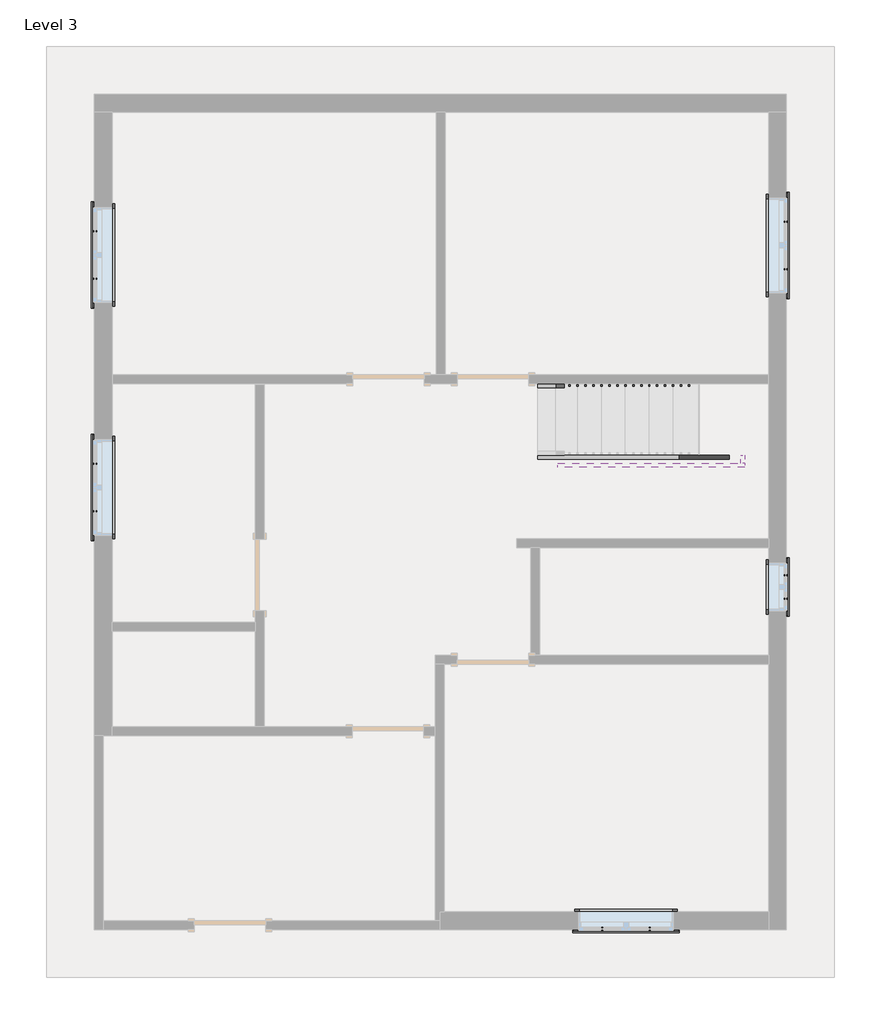
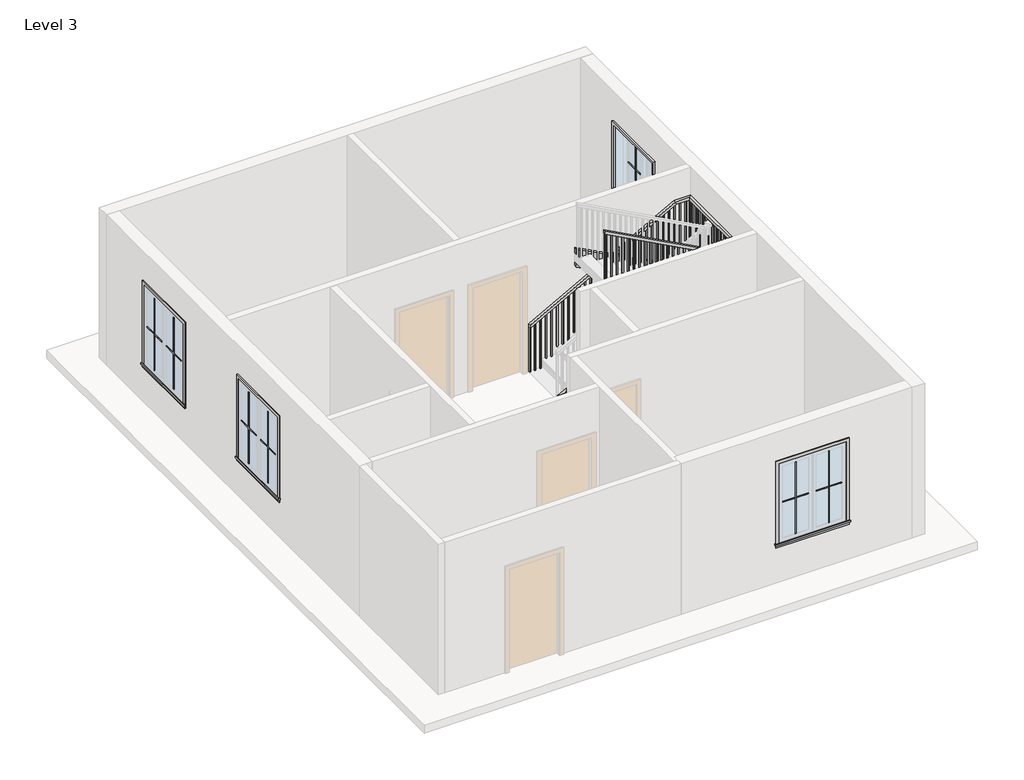
# One storey, part 2 of 2: 20 proxies, 3 members, 1 railing.
"""IFC4 building model written with IfcOpenShell, lengths in millimetres."""

from ifc_helpers import new_model, si_unit, frame, origin, place, context, project, spatial, polyline, outline, extrude, faceted_brep, transform, mapped, element, save
from components import muntin_pattern_2x2_muntin_pattern_2x2_6dad3731, muntin_pattern_2x2_muntin_pattern_2x2_a30a3345, muntin_pattern_2x2_muntin_pattern_2x2_53152e2c, muntin_pattern_2x2_muntin_pattern_2x2_e8f3e573, trim_window_exterior_flat_with_sill_92b9b949, trim_window_exterior_flat_with_sill_a665a915, trim_window_interior_flat_picture_frame_3bb882cf, trim_window_interior_flat_picture_frame_d485c387

model = new_model("IFC4")

# Units and contexts
model_context = context("Model", 3, world=origin())
ifc_project = project(units=[si_unit("LENGTHUNIT", "METRE", prefix="MILLI")], contexts=[model_context])

# Site, building, storey
site = spatial("IfcSite", under=ifc_project)
building = spatial("IfcBuilding", under=site)
storey = spatial("IfcBuildingStorey", under=building, Name="Level 3", Elevation=6096.0)

# Proxies
placement = place(None, origin())
muntin_pattern_2x2_muntin_pattern_2x2_shape = muntin_pattern_2x2_muntin_pattern_2x2_6dad3731(model_context)
element("IfcBuildingElementProxy", 1, Name="Muntin Pattern_2x2 : Muntin Pattern_2x2", ObjectType="Muntin Pattern_2x2 : Muntin Pattern_2x2", at=placement, inside=storey, context=model_context, shape_type="MappedRepresentation", body=[
    mapped(muntin_pattern_2x2_muntin_pattern_2x2_shape, transform((10003.63125, 2232.025, 7080.25), x_axis=(-1.0, 0.0, 0.0), y_axis=(0.0, -1.0, 0.0), z_axis=(0.0, 0.0, 1.0))),
])
element("IfcBuildingElementProxy", 2, Name="Muntin Pattern_2x2 : Muntin Pattern_2x2", ObjectType="Muntin Pattern_2x2 : Muntin Pattern_2x2", at=placement, inside=storey, context=model_context, shape_type="MappedRepresentation", body=[
    mapped(muntin_pattern_2x2_muntin_pattern_2x2_shape, transform((2917.825, 7567.6125, 7080.25), x_axis=(0.0, 1.0, 0.0), y_axis=(-1.0, 0.0, 0.0), z_axis=(0.0, 0.0, 1.0))),
])
element("IfcBuildingElementProxy", 3, Name="Muntin Pattern_2x2 : Muntin Pattern_2x2", ObjectType="Muntin Pattern_2x2 : Muntin Pattern_2x2", at=placement, inside=storey, context=model_context, shape_type="MappedRepresentation", body=[
    mapped(muntin_pattern_2x2_muntin_pattern_2x2_shape, transform((2917.825, 10536.2375, 7080.25), x_axis=(0.0, 1.0, 0.0), y_axis=(-1.0, 0.0, 0.0), z_axis=(0.0, 0.0, 1.0))),
])
element("IfcBuildingElementProxy", 4, Name="Muntin Pattern_2x2 : Muntin Pattern_2x2", ObjectType="Muntin Pattern_2x2 : Muntin Pattern_2x2", at=placement, inside=storey, context=model_context, shape_type="MappedRepresentation", body=[
    mapped(muntin_pattern_2x2_muntin_pattern_2x2_shape, transform((11737.975, 11264.9, 7080.25), x_axis=(0.0, -1.0, 0.0), y_axis=(1.0, 0.0, 0.0), z_axis=(0.0, 0.0, 1.0))),
])
muntin_pattern_2x2_muntin_pattern_2x2_2_shape = muntin_pattern_2x2_muntin_pattern_2x2_a30a3345(model_context)
element("IfcBuildingElementProxy", 5, Name="Muntin Pattern_2x2 : Muntin Pattern_2x2", ObjectType="Muntin Pattern_2x2 : Muntin Pattern_2x2", at=placement, inside=storey, context=model_context, shape_type="MappedRepresentation", body=[
    mapped(muntin_pattern_2x2_muntin_pattern_2x2_2_shape, transform((9397.20625, 2232.025, 7080.25), x_axis=(1.0, 0.0, 0.0), y_axis=(0.0, 1.0, 0.0), z_axis=(0.0, 0.0, 1.0))),
])
element("IfcBuildingElementProxy", 6, Name="Muntin Pattern_2x2 : Muntin Pattern_2x2", ObjectType="Muntin Pattern_2x2 : Muntin Pattern_2x2", at=placement, inside=storey, context=model_context, shape_type="MappedRepresentation", body=[
    mapped(muntin_pattern_2x2_muntin_pattern_2x2_2_shape, transform((2917.825, 8174.0375, 7080.25), x_axis=(0.0, -1.0, 0.0), y_axis=(1.0, 0.0, 0.0), z_axis=(0.0, 0.0, 1.0))),
])
element("IfcBuildingElementProxy", 7, Name="Muntin Pattern_2x2 : Muntin Pattern_2x2", ObjectType="Muntin Pattern_2x2 : Muntin Pattern_2x2", at=placement, inside=storey, context=model_context, shape_type="MappedRepresentation", body=[
    mapped(muntin_pattern_2x2_muntin_pattern_2x2_2_shape, transform((2917.825, 11142.6625, 7080.25), x_axis=(0.0, -1.0, 0.0), y_axis=(1.0, 0.0, 0.0), z_axis=(0.0, 0.0, 1.0))),
])
element("IfcBuildingElementProxy", 8, Name="Muntin Pattern_2x2 : Muntin Pattern_2x2", ObjectType="Muntin Pattern_2x2 : Muntin Pattern_2x2", at=placement, inside=storey, context=model_context, shape_type="MappedRepresentation", body=[
    mapped(muntin_pattern_2x2_muntin_pattern_2x2_2_shape, transform((11737.975, 10658.475, 7080.25), x_axis=(0.0, 1.0, 0.0), y_axis=(-1.0, 0.0, 0.0), z_axis=(0.0, 0.0, 1.0))),
])
muntin_pattern_2x2_muntin_pattern_2x2_3_shape = muntin_pattern_2x2_muntin_pattern_2x2_53152e2c(model_context)
element("IfcBuildingElementProxy", 9, Name="Muntin Pattern_2x2 : Muntin Pattern_2x2", ObjectType="Muntin Pattern_2x2 : Muntin Pattern_2x2", at=placement, inside=storey, context=model_context, shape_type="MappedRepresentation", body=[
    mapped(muntin_pattern_2x2_muntin_pattern_2x2_3_shape, transform((11737.975, 6748.4625, 7080.25), x_axis=(0.0, -1.0, 0.0), y_axis=(1.0, 0.0, 0.0), z_axis=(0.0, 0.0, 1.0))),
])
muntin_pattern_2x2_muntin_pattern_2x2_4_shape = muntin_pattern_2x2_muntin_pattern_2x2_e8f3e573(model_context)
element("IfcBuildingElementProxy", 10, Name="Muntin Pattern_2x2 : Muntin Pattern_2x2", ObjectType="Muntin Pattern_2x2 : Muntin Pattern_2x2", at=placement, inside=storey, context=model_context, shape_type="MappedRepresentation", body=[
    mapped(muntin_pattern_2x2_muntin_pattern_2x2_4_shape, transform((11737.975, 6446.8375, 7080.25), x_axis=(0.0, 1.0, 0.0), y_axis=(-1.0, 0.0, 0.0), z_axis=(0.0, 0.0, 1.0))),
])
trim_window_exterior_flat_with_sill_shape = trim_window_exterior_flat_with_sill_92b9b949(model_context)
element("IfcBuildingElementProxy", 11, Name="Trim-Window-Exterior-Flat : with Sill", ObjectType="Trim-Window-Exterior-Flat : with Sill", at=placement, inside=storey, context=model_context, shape_type="MappedRepresentation", body=[
    mapped(trim_window_exterior_flat_with_sill_shape, transform((9700.41875, 2222.5, 8534.4), x_axis=(1.0, 0.0, 0.0), y_axis=(0.0, 0.0, 1.0), z_axis=(0.0, -1.0, 0.0))),
])
element("IfcBuildingElementProxy", 12, Name="Trim-Window-Exterior-Flat : with Sill", ObjectType="Trim-Window-Exterior-Flat : with Sill", at=placement, inside=storey, context=model_context, shape_type="MappedRepresentation", body=[
    mapped(trim_window_exterior_flat_with_sill_shape, transform((2908.3, 7870.825, 8534.4), x_axis=(0.0, -1.0, 0.0), y_axis=(0.0, 0.0, 1.0), z_axis=(-1.0, 0.0, 0.0))),
])
element("IfcBuildingElementProxy", 13, Name="Trim-Window-Exterior-Flat : with Sill", ObjectType="Trim-Window-Exterior-Flat : with Sill", at=placement, inside=storey, context=model_context, shape_type="MappedRepresentation", body=[
    mapped(trim_window_exterior_flat_with_sill_shape, transform((2908.3, 10839.45, 8534.4), x_axis=(0.0, -1.0, 0.0), y_axis=(0.0, 0.0, 1.0), z_axis=(-1.0, 0.0, 0.0))),
])
element("IfcBuildingElementProxy", 14, Name="Trim-Window-Exterior-Flat : with Sill", ObjectType="Trim-Window-Exterior-Flat : with Sill", at=placement, inside=storey, context=model_context, shape_type="MappedRepresentation", body=[
    mapped(trim_window_exterior_flat_with_sill_shape, transform((11747.5, 10961.6875, 8534.4), x_axis=(0.0, 1.0, 0.0), y_axis=(0.0, 0.0, 1.0), z_axis=(1.0, 0.0, 0.0))),
])
trim_window_exterior_flat_with_sill_2_shape = trim_window_exterior_flat_with_sill_a665a915(model_context)
element("IfcBuildingElementProxy", 15, Name="Trim-Window-Exterior-Flat : with Sill", ObjectType="Trim-Window-Exterior-Flat : with Sill", at=placement, inside=storey, context=model_context, shape_type="MappedRepresentation", body=[
    mapped(trim_window_exterior_flat_with_sill_2_shape, transform((11747.5, 6597.65, 7924.8), x_axis=(0.0, 1.0, 0.0), y_axis=(0.0, 0.0, 1.0), z_axis=(1.0, 0.0, 0.0))),
])
trim_window_interior_flat_picture_frame_shape = trim_window_interior_flat_picture_frame_3bb882cf(model_context)
element("IfcBuildingElementProxy", 16, Name="Trim-Window-Interior-Flat : Picture Frame", ObjectType="Trim-Window-Interior-Flat : Picture Frame", at=placement, inside=storey, context=model_context, shape_type="MappedRepresentation", body=[
    mapped(trim_window_interior_flat_picture_frame_shape, transform((9700.41875, 2451.1, 8534.4), x_axis=(-1.0, 0.0, 0.0), y_axis=(0.0, 0.0, 1.0), z_axis=(0.0, 1.0, 0.0))),
])
element("IfcBuildingElementProxy", 17, Name="Trim-Window-Interior-Flat : Picture Frame", ObjectType="Trim-Window-Interior-Flat : Picture Frame", at=placement, inside=storey, context=model_context, shape_type="MappedRepresentation", body=[
    mapped(trim_window_interior_flat_picture_frame_shape, transform((3136.9, 7870.825, 8534.4), x_axis=(0.0, 1.0, 0.0), y_axis=(0.0, 0.0, 1.0), z_axis=(1.0, 0.0, 0.0))),
])
element("IfcBuildingElementProxy", 18, Name="Trim-Window-Interior-Flat : Picture Frame", ObjectType="Trim-Window-Interior-Flat : Picture Frame", at=placement, inside=storey, context=model_context, shape_type="MappedRepresentation", body=[
    mapped(trim_window_interior_flat_picture_frame_shape, transform((3136.9, 10839.45, 8534.4), x_axis=(0.0, 1.0, 0.0), y_axis=(0.0, 0.0, 1.0), z_axis=(1.0, 0.0, 0.0))),
])
element("IfcBuildingElementProxy", 19, Name="Trim-Window-Interior-Flat : Picture Frame", ObjectType="Trim-Window-Interior-Flat : Picture Frame", at=placement, inside=storey, context=model_context, shape_type="MappedRepresentation", body=[
    mapped(trim_window_interior_flat_picture_frame_shape, transform((11518.9, 10961.6875, 8534.4), x_axis=(0.0, -1.0, 0.0), y_axis=(0.0, 0.0, 1.0), z_axis=(-1.0, 0.0, 0.0))),
])
trim_window_interior_flat_picture_frame_2_shape = trim_window_interior_flat_picture_frame_d485c387(model_context)
element("IfcBuildingElementProxy", 20, Name="Trim-Window-Interior-Flat : Picture Frame", ObjectType="Trim-Window-Interior-Flat : Picture Frame", at=placement, inside=storey, context=model_context, shape_type="MappedRepresentation", body=[
    mapped(trim_window_interior_flat_picture_frame_2_shape, transform((11518.9, 6597.65, 7924.8), x_axis=(0.0, -1.0, 0.0), y_axis=(0.0, 0.0, 1.0), z_axis=(-1.0, 0.0, 0.0))),
])

# Members
element("IfcMember", 21, ObjectType="Stringer - 2\" Width", at=placement, inside=storey, context=model_context, shape_type="SweptSolid", body=[
    extrude(outline(polyline([(6340.4581083, 8572.5), (6096.0, 8572.5), (6096.0, 8761.9689927), (7373.1621978, 11163.3), (7718.3905183, 11163.3), (6340.4581083, 8572.5)])), frame((0.0, 8229.6, 0.0), z_axis=(0.0, 1.0, 0.0), x_axis=(0.0, 0.0, 1.0)), (0.0, 0.0, 1.0), 50.8),
])
element("IfcMember", 22, ObjectType="Stringer - 2\" Width", at=placement, inside=storey, context=model_context, shape_type="SweptSolid", body=[
    extrude(outline(polyline([(11163.3, 8280.4), (11214.1, 8280.4), (11214.1, 8178.8), (11163.3, 8178.8), (11163.3, 8280.4)])), frame((0.0, 0.0, 7471.6105263), z_axis=(0.0, 0.0, 1.0), x_axis=(1.0, 0.0, 0.0)), (0.0, 0.0, 1.0), 304.8),
])
element("IfcMember", 23, ObjectType="Stringer - 2\" Width", at=placement, inside=storey, context=model_context, shape_type="SweptSolid", body=[
    extrude(outline(polyline([(7560.9419568, 11214.1), (7905.380564, 11214.1), (9162.012143, 8826.5), (8817.5735358, 8826.5), (7560.9419568, 11214.1)])), frame((0.0, 8128.0, 0.0), z_axis=(0.0, 1.0, 0.0), x_axis=(0.0, 0.0, 1.0)), (0.0, 0.0, 1.0), 50.8),
])

# Railing
element("IfcRailing", 24, ObjectType="Handrail - Rectangular", at=placement, inside=storey, context=model_context, shape_type="SolidModel", body=[
    faceted_brep([(8572.5, 9194.8, 7170.8210526), (8572.5, 9194.8, 7112.9285199), (8572.5, 9144.0, 7112.9285199), (8572.5, 9144.0, 7170.8210526), (11214.1, 9194.8, 8614.6105263), (11227.076708, 9194.8, 8563.8105263), (11227.076708, 9144.0, 8563.8105263), (11214.1, 9144.0, 8614.6105263), (11518.9, 9194.8, 8614.6105263), (11518.9, 9194.8, 8563.8105263), (11468.1, 9144.0, 8563.8105263), (11468.1, 9144.0, 8614.6105263), (11518.9, 7340.6, 8614.6105263), (11518.9, 7289.8, 8563.8105263), (11468.1, 7289.8, 8563.8105263), (11468.1, 7340.6, 8614.6105263), (11518.9, 7340.6, 8679.4615901), (11518.9, 7289.8, 8628.6615901), (11468.1, 7289.8, 8628.6615901), (11468.1, 7340.6, 8679.4615901), (11518.9, 7213.6, 8679.4615901), (11518.9, 7213.6, 8628.6615901), (11468.1, 7264.4, 8628.6615901), (11468.1, 7264.4, 8679.4615901), (11391.9, 7213.6, 8679.4615901), (11379.1122768, 7213.6, 8628.6615901), (11379.1122768, 7264.4, 8628.6615901), (11391.9, 7264.4, 8679.4615901), (8826.5, 7213.6, 10058.4), (8826.5, 7264.4, 10058.4), (8826.5, 7264.4, 10000.7264198), (8826.5, 7213.6, 10000.7264198)], [[[0, 1, 2, 3]], [[1, 0, 4, 5]], [[2, 1, 5, 6]], [[3, 2, 6, 7]], [[0, 3, 7, 4]], [[5, 4, 8, 9]], [[6, 5, 9, 10]], [[7, 6, 10, 11]], [[4, 7, 11, 8]], [[9, 8, 12, 13]], [[10, 9, 13, 14]], [[11, 10, 14, 15]], [[8, 11, 15, 12]], [[13, 12, 16, 17]], [[14, 13, 17, 18]], [[15, 14, 18, 19]], [[12, 15, 19, 16]], [[17, 16, 20, 21]], [[18, 17, 21, 22]], [[19, 18, 22, 23]], [[16, 19, 23, 20]], [[21, 20, 24, 25]], [[22, 21, 25, 26]], [[23, 22, 26, 27]], [[20, 23, 27, 24]], [[28, 29, 30, 31]], [[25, 24, 28, 31]], [[26, 25, 31, 30]], [[27, 26, 30, 29]], [[24, 27, 29, 28]]]),
    extrude(outline(polyline([(9992.193385, 8842.375), (8983.5789474, 8842.375), (8983.5789474, 8861.425), (9981.9537434, 8861.425), (9992.193385, 8842.375)])), frame((0.0, 7229.475, 0.0), z_axis=(0.0, 1.0, 0.0), x_axis=(0.0, 0.0, 1.0)), (0.0, 0.0, 1.0), 19.05),
    extrude(outline(polyline([(9937.5819629, 8943.975), (8983.5789474, 8943.975), (8983.5789474, 8963.025), (9927.3423212, 8963.025), (9937.5819629, 8943.975)])), frame((0.0, 7229.475, 0.0), z_axis=(0.0, 1.0, 0.0), x_axis=(0.0, 0.0, 1.0)), (0.0, 0.0, 1.0), 19.05),
    extrude(outline(polyline([(9882.9705407, 9045.575), (8983.5789474, 9045.575), (8983.5789474, 9064.625), (9872.730899, 9064.625), (9882.9705407, 9045.575)])), frame((0.0, 7229.475, 0.0), z_axis=(0.0, 1.0, 0.0), x_axis=(0.0, 0.0, 1.0)), (0.0, 0.0, 1.0), 19.05),
    extrude(outline(polyline([(9828.3591185, 9147.175), (8823.1578947, 9147.175), (8823.1578947, 9166.225), (9818.1194769, 9166.225), (9828.3591185, 9147.175)])), frame((0.0, 7229.475, 0.0), z_axis=(0.0, 1.0, 0.0), x_axis=(0.0, 0.0, 1.0)), (0.0, 0.0, 1.0), 19.05),
    extrude(outline(polyline([(9773.7476964, 9248.775), (8823.1578947, 9248.775), (8823.1578947, 9267.825), (9763.5080547, 9267.825), (9773.7476964, 9248.775)])), frame((0.0, 7229.475, 0.0), z_axis=(0.0, 1.0, 0.0), x_axis=(0.0, 0.0, 1.0)), (0.0, 0.0, 1.0), 19.05),
    extrude(outline(polyline([(9719.1362742, 9350.375), (8823.1578947, 9350.375), (8823.1578947, 9369.425), (9708.8966325, 9369.425), (9719.1362742, 9350.375)])), frame((0.0, 7229.475, 0.0), z_axis=(0.0, 1.0, 0.0), x_axis=(0.0, 0.0, 1.0)), (0.0, 0.0, 1.0), 19.05),
    extrude(outline(polyline([(9664.524852, 9451.975), (8662.7368421, 9451.975), (8662.7368421, 9471.025), (9654.2852104, 9471.025), (9664.524852, 9451.975)])), frame((0.0, 7229.475, 0.0), z_axis=(0.0, 1.0, 0.0), x_axis=(0.0, 0.0, 1.0)), (0.0, 0.0, 1.0), 19.05),
    extrude(outline(polyline([(9609.9134298, 9553.575), (8662.7368421, 9553.575), (8662.7368421, 9572.625), (9599.6737882, 9572.625), (9609.9134298, 9553.575)])), frame((0.0, 7229.475, 0.0), z_axis=(0.0, 1.0, 0.0), x_axis=(0.0, 0.0, 1.0)), (0.0, 0.0, 1.0), 19.05),
    extrude(outline(polyline([(9555.3004835, 9655.175), (8662.7368421, 9655.175), (8662.7368421, 9674.225), (9544.8885402, 9674.225), (9555.3004835, 9655.175)])), frame((0.0, 7229.475, 0.0), z_axis=(0.0, 1.0, 0.0), x_axis=(0.0, 0.0, 1.0)), (0.0, 0.0, 1.0), 19.05),
    extrude(outline(polyline([(9500.6905855, 9756.775), (8502.3157895, 9756.775), (8502.3157895, 9775.825), (9490.4509438, 9775.825), (9500.6905855, 9756.775)])), frame((0.0, 7229.475, 0.0), z_axis=(0.0, 1.0, 0.0), x_axis=(0.0, 0.0, 1.0)), (0.0, 0.0, 1.0), 19.05),
    extrude(outline(polyline([(9446.0791633, 9858.375), (8502.3157895, 9858.375), (8502.3157895, 9877.425), (9435.8395217, 9877.425), (9446.0791633, 9858.375)])), frame((0.0, 7229.475, 0.0), z_axis=(0.0, 1.0, 0.0), x_axis=(0.0, 0.0, 1.0)), (0.0, 0.0, 1.0), 19.05),
    extrude(outline(polyline([(9391.4677411, 9959.975), (8502.3157895, 9959.975), (8502.3157895, 9979.025), (9381.2280995, 9979.025), (9391.4677411, 9959.975)])), frame((0.0, 7229.475, 0.0), z_axis=(0.0, 1.0, 0.0), x_axis=(0.0, 0.0, 1.0)), (0.0, 0.0, 1.0), 19.05),
    extrude(outline(polyline([(9336.856319, 10061.575), (8341.8947368, 10061.575), (8341.8947368, 10080.625), (9326.6166773, 10080.625), (9336.856319, 10061.575)])), frame((0.0, 7229.475, 0.0), z_axis=(0.0, 1.0, 0.0), x_axis=(0.0, 0.0, 1.0)), (0.0, 0.0, 1.0), 19.05),
    extrude(outline(polyline([(9282.2448968, 10163.175), (8341.8947368, 10163.175), (8341.8947368, 10182.225), (9272.0052551, 10182.225), (9282.2448968, 10163.175)])), frame((0.0, 7229.475, 0.0), z_axis=(0.0, 1.0, 0.0), x_axis=(0.0, 0.0, 1.0)), (0.0, 0.0, 1.0), 19.05),
    extrude(outline(polyline([(9227.6334746, 10264.775), (8341.8947368, 10264.775), (8341.8947368, 10283.825), (9217.393833, 10283.825), (9227.6334746, 10264.775)])), frame((0.0, 7229.475, 0.0), z_axis=(0.0, 1.0, 0.0), x_axis=(0.0, 0.0, 1.0)), (0.0, 0.0, 1.0), 19.05),
    extrude(outline(polyline([(9173.0220525, 10366.375), (8181.4736842, 10366.375), (8181.4736842, 10385.425), (9162.7824108, 10385.425), (9173.0220525, 10366.375)])), frame((0.0, 7229.475, 0.0), z_axis=(0.0, 1.0, 0.0), x_axis=(0.0, 0.0, 1.0)), (0.0, 0.0, 1.0), 19.05),
    extrude(outline(polyline([(9118.4106303, 10467.975), (8181.4736842, 10467.975), (8181.4736842, 10487.025), (9108.1709886, 10487.025), (9118.4106303, 10467.975)])), frame((0.0, 7229.475, 0.0), z_axis=(0.0, 1.0, 0.0), x_axis=(0.0, 0.0, 1.0)), (0.0, 0.0, 1.0), 19.05),
    extrude(outline(polyline([(9063.7992081, 10569.575), (8181.4736842, 10569.575), (8181.4736842, 10588.625), (9053.5595665, 10588.625), (9063.7992081, 10569.575)])), frame((0.0, 7229.475, 0.0), z_axis=(0.0, 1.0, 0.0), x_axis=(0.0, 0.0, 1.0)), (0.0, 0.0, 1.0), 19.05),
    extrude(outline(polyline([(9009.1877859, 10671.175), (8021.0526316, 10671.175), (8021.0526316, 10690.225), (8998.9481443, 10690.225), (9009.1877859, 10671.175)])), frame((0.0, 7229.475, 0.0), z_axis=(0.0, 1.0, 0.0), x_axis=(0.0, 0.0, 1.0)), (0.0, 0.0, 1.0), 19.05),
    extrude(outline(polyline([(8954.5763638, 10772.775), (8021.0526316, 10772.775), (8021.0526316, 10791.825), (8944.3367221, 10791.825), (8954.5763638, 10772.775)])), frame((0.0, 7229.475, 0.0), z_axis=(0.0, 1.0, 0.0), x_axis=(0.0, 0.0, 1.0)), (0.0, 0.0, 1.0), 19.05),
    extrude(outline(polyline([(8899.9649416, 10874.375), (8021.0526316, 10874.375), (8021.0526316, 10893.425), (8889.7252999, 10893.425), (8899.9649416, 10874.375)])), frame((0.0, 7229.475, 0.0), z_axis=(0.0, 1.0, 0.0), x_axis=(0.0, 0.0, 1.0)), (0.0, 0.0, 1.0), 19.05),
    extrude(outline(polyline([(8845.3535194, 10975.975), (7860.6315789, 10975.975), (7860.6315789, 10995.025), (8835.1138778, 10995.025), (8845.3535194, 10975.975)])), frame((0.0, 7229.475, 0.0), z_axis=(0.0, 1.0, 0.0), x_axis=(0.0, 0.0, 1.0)), (0.0, 0.0, 1.0), 19.05),
    extrude(outline(polyline([(8790.7420972, 11077.575), (7860.6315789, 11077.575), (7860.6315789, 11096.625), (8780.5024556, 11096.625), (8790.7420972, 11077.575)])), frame((0.0, 7229.475, 0.0), z_axis=(0.0, 1.0, 0.0), x_axis=(0.0, 0.0, 1.0)), (0.0, 0.0, 1.0), 19.05),
    extrude(outline(polyline([(8736.1306751, 11179.175), (7860.6315789, 11179.175), (7860.6315789, 11198.225), (8725.8910334, 11198.225), (8736.1306751, 11179.175)])), frame((0.0, 7229.475, 0.0), z_axis=(0.0, 1.0, 0.0), x_axis=(0.0, 0.0, 1.0)), (0.0, 0.0, 1.0), 19.05),
    extrude(outline(polyline([(8681.5192529, 11280.775), (7700.2105263, 11280.775), (7700.2105263, 11299.825), (8671.2796112, 11299.825), (8681.5192529, 11280.775)])), frame((0.0, 7229.475, 0.0), z_axis=(0.0, 1.0, 0.0), x_axis=(0.0, 0.0, 1.0)), (0.0, 0.0, 1.0), 19.05),
    extrude(outline(polyline([(8626.9078307, 11382.375), (7700.2105263, 11382.375), (7700.2105263, 11401.425), (8616.6681891, 11401.425), (8626.9078307, 11382.375)])), frame((0.0, 7229.475, 0.0), z_axis=(0.0, 1.0, 0.0), x_axis=(0.0, 0.0, 1.0)), (0.0, 0.0, 1.0), 19.05),
    extrude(outline(polyline([(11503.025, 7350.125), (11503.025, 7331.075), (11483.975, 7331.075), (11483.975, 7350.125), (11503.025, 7350.125)])), frame((0.0, 0.0, 7700.2105263), z_axis=(0.0, 0.0, 1.0), x_axis=(1.0, 0.0, 0.0)), (0.0, 0.0, 1.0), 863.6),
    extrude(outline(polyline([(11503.025, 7451.725), (11503.025, 7432.675), (11483.975, 7432.675), (11483.975, 7451.725), (11503.025, 7451.725)])), frame((0.0, 0.0, 7700.2105263), z_axis=(0.0, 0.0, 1.0), x_axis=(1.0, 0.0, 0.0)), (0.0, 0.0, 1.0), 863.6),
    extrude(outline(polyline([(11503.025, 7553.325), (11503.025, 7534.275), (11483.975, 7534.275), (11483.975, 7553.325), (11503.025, 7553.325)])), frame((0.0, 0.0, 7700.2105263), z_axis=(0.0, 0.0, 1.0), x_axis=(1.0, 0.0, 0.0)), (0.0, 0.0, 1.0), 863.6),
    extrude(outline(polyline([(11503.025, 7654.925), (11503.025, 7635.875), (11483.975, 7635.875), (11483.975, 7654.925), (11503.025, 7654.925)])), frame((0.0, 0.0, 7700.2105263), z_axis=(0.0, 0.0, 1.0), x_axis=(1.0, 0.0, 0.0)), (0.0, 0.0, 1.0), 863.6),
    extrude(outline(polyline([(11503.025, 7756.525), (11503.025, 7737.475), (11483.975, 7737.475), (11483.975, 7756.525), (11503.025, 7756.525)])), frame((0.0, 0.0, 7700.2105263), z_axis=(0.0, 0.0, 1.0), x_axis=(1.0, 0.0, 0.0)), (0.0, 0.0, 1.0), 863.6),
    extrude(outline(polyline([(11503.025, 7858.125), (11503.025, 7839.075), (11483.975, 7839.075), (11483.975, 7858.125), (11503.025, 7858.125)])), frame((0.0, 0.0, 7700.2105263), z_axis=(0.0, 0.0, 1.0), x_axis=(1.0, 0.0, 0.0)), (0.0, 0.0, 1.0), 863.6),
    extrude(outline(polyline([(11503.025, 7959.725), (11503.025, 7940.675), (11483.975, 7940.675), (11483.975, 7959.725), (11503.025, 7959.725)])), frame((0.0, 0.0, 7700.2105263), z_axis=(0.0, 0.0, 1.0), x_axis=(1.0, 0.0, 0.0)), (0.0, 0.0, 1.0), 863.6),
    extrude(outline(polyline([(11503.025, 8061.325), (11503.025, 8042.275), (11483.975, 8042.275), (11483.975, 8061.325), (11503.025, 8061.325)])), frame((0.0, 0.0, 7700.2105263), z_axis=(0.0, 0.0, 1.0), x_axis=(1.0, 0.0, 0.0)), (0.0, 0.0, 1.0), 863.6),
    extrude(outline(polyline([(11503.025, 8162.925), (11503.025, 8143.875), (11483.975, 8143.875), (11483.975, 8162.925), (11503.025, 8162.925)])), frame((0.0, 0.0, 7700.2105263), z_axis=(0.0, 0.0, 1.0), x_axis=(1.0, 0.0, 0.0)), (0.0, 0.0, 1.0), 863.6),
    extrude(outline(polyline([(11503.025, 8264.525), (11503.025, 8245.475), (11483.975, 8245.475), (11483.975, 8264.525), (11503.025, 8264.525)])), frame((0.0, 0.0, 7700.2105263), z_axis=(0.0, 0.0, 1.0), x_axis=(1.0, 0.0, 0.0)), (0.0, 0.0, 1.0), 863.6),
    extrude(outline(polyline([(11503.025, 8366.125), (11503.025, 8347.075), (11483.975, 8347.075), (11483.975, 8366.125), (11503.025, 8366.125)])), frame((0.0, 0.0, 7700.2105263), z_axis=(0.0, 0.0, 1.0), x_axis=(1.0, 0.0, 0.0)), (0.0, 0.0, 1.0), 863.6),
    extrude(outline(polyline([(11503.025, 8467.725), (11503.025, 8448.675), (11483.975, 8448.675), (11483.975, 8467.725), (11503.025, 8467.725)])), frame((0.0, 0.0, 7700.2105263), z_axis=(0.0, 0.0, 1.0), x_axis=(1.0, 0.0, 0.0)), (0.0, 0.0, 1.0), 863.6),
    extrude(outline(polyline([(11503.025, 8569.325), (11503.025, 8550.275), (11483.975, 8550.275), (11483.975, 8569.325), (11503.025, 8569.325)])), frame((0.0, 0.0, 7700.2105263), z_axis=(0.0, 0.0, 1.0), x_axis=(1.0, 0.0, 0.0)), (0.0, 0.0, 1.0), 863.6),
    extrude(outline(polyline([(11503.025, 8670.925), (11503.025, 8651.875), (11483.975, 8651.875), (11483.975, 8670.925), (11503.025, 8670.925)])), frame((0.0, 0.0, 7700.2105263), z_axis=(0.0, 0.0, 1.0), x_axis=(1.0, 0.0, 0.0)), (0.0, 0.0, 1.0), 863.6),
    extrude(outline(polyline([(11503.025, 8772.525), (11503.025, 8753.475), (11483.975, 8753.475), (11483.975, 8772.525), (11503.025, 8772.525)])), frame((0.0, 0.0, 7700.2105263), z_axis=(0.0, 0.0, 1.0), x_axis=(1.0, 0.0, 0.0)), (0.0, 0.0, 1.0), 863.6),
    extrude(outline(polyline([(11503.025, 8874.125), (11503.025, 8855.075), (11483.975, 8855.075), (11483.975, 8874.125), (11503.025, 8874.125)])), frame((0.0, 0.0, 7700.2105263), z_axis=(0.0, 0.0, 1.0), x_axis=(1.0, 0.0, 0.0)), (0.0, 0.0, 1.0), 863.6),
    extrude(outline(polyline([(11503.025, 8975.725), (11503.025, 8956.675), (11483.975, 8956.675), (11483.975, 8975.725), (11503.025, 8975.725)])), frame((0.0, 0.0, 7700.2105263), z_axis=(0.0, 0.0, 1.0), x_axis=(1.0, 0.0, 0.0)), (0.0, 0.0, 1.0), 863.6),
    extrude(outline(polyline([(11503.025, 9077.325), (11503.025, 9058.275), (11483.975, 9058.275), (11483.975, 9077.325), (11503.025, 9077.325)])), frame((0.0, 0.0, 7700.2105263), z_axis=(0.0, 0.0, 1.0), x_axis=(1.0, 0.0, 0.0)), (0.0, 0.0, 1.0), 863.6),
    extrude(outline(polyline([(11407.775, 9178.925), (11426.825, 9178.925), (11426.825, 9159.875), (11407.775, 9159.875), (11407.775, 9178.925)])), frame((0.0, 0.0, 7700.2105263), z_axis=(0.0, 0.0, 1.0), x_axis=(1.0, 0.0, 0.0)), (0.0, 0.0, 1.0), 863.6),
    extrude(outline(polyline([(11306.175, 9178.925), (11325.225, 9178.925), (11325.225, 9159.875), (11306.175, 9159.875), (11306.175, 9178.925)])), frame((0.0, 0.0, 7700.2105263), z_axis=(0.0, 0.0, 1.0), x_axis=(1.0, 0.0, 0.0)), (0.0, 0.0, 1.0), 863.6),
    extrude(outline(polyline([(8551.512022, 11204.575), (7700.2105263, 11204.575), (7700.2105263, 11223.625), (8561.9239653, 11223.625), (8551.512022, 11204.575)])), frame((0.0, 9159.875, 0.0), z_axis=(0.0, 1.0, 0.0), x_axis=(0.0, 0.0, 1.0)), (0.0, 0.0, 1.0), 19.05),
    extrude(outline(polyline([(8495.9816576, 11102.975), (7539.7894737, 11102.975), (7539.7894737, 11122.025), (8506.3936009, 11122.025), (8495.9816576, 11102.975)])), frame((0.0, 9159.875, 0.0), z_axis=(0.0, 1.0, 0.0), x_axis=(0.0, 0.0, 1.0)), (0.0, 0.0, 1.0), 19.05),
    extrude(outline(polyline([(8440.4512932, 11001.375), (7539.7894737, 11001.375), (7539.7894737, 11020.425), (8450.8632365, 11020.425), (8440.4512932, 11001.375)])), frame((0.0, 9159.875, 0.0), z_axis=(0.0, 1.0, 0.0), x_axis=(0.0, 0.0, 1.0)), (0.0, 0.0, 1.0), 19.05),
    extrude(outline(polyline([(8384.9209288, 10899.775), (7539.7894737, 10899.775), (7539.7894737, 10918.825), (8395.3328722, 10918.825), (8384.9209288, 10899.775)])), frame((0.0, 9159.875, 0.0), z_axis=(0.0, 1.0, 0.0), x_axis=(0.0, 0.0, 1.0)), (0.0, 0.0, 1.0), 19.05),
    extrude(outline(polyline([(8329.3905645, 10798.175), (7379.3684211, 10798.175), (7379.3684211, 10817.225), (8339.8025078, 10817.225), (8329.3905645, 10798.175)])), frame((0.0, 9159.875, 0.0), z_axis=(0.0, 1.0, 0.0), x_axis=(0.0, 0.0, 1.0)), (0.0, 0.0, 1.0), 19.05),
    extrude(outline(polyline([(8273.8602001, 10696.575), (7379.3684211, 10696.575), (7379.3684211, 10715.625), (8284.2721434, 10715.625), (8273.8602001, 10696.575)])), frame((0.0, 9159.875, 0.0), z_axis=(0.0, 1.0, 0.0), x_axis=(0.0, 0.0, 1.0)), (0.0, 0.0, 1.0), 19.05),
    extrude(outline(polyline([(8218.3298357, 10594.975), (7379.3684211, 10594.975), (7379.3684211, 10614.025), (8228.741779, 10614.025), (8218.3298357, 10594.975)])), frame((0.0, 9159.875, 0.0), z_axis=(0.0, 1.0, 0.0), x_axis=(0.0, 0.0, 1.0)), (0.0, 0.0, 1.0), 19.05),
    extrude(outline(polyline([(8162.7994714, 10493.375), (7218.9473684, 10493.375), (7218.9473684, 10512.425), (8173.2114147, 10512.425), (8162.7994714, 10493.375)])), frame((0.0, 9159.875, 0.0), z_axis=(0.0, 1.0, 0.0), x_axis=(0.0, 0.0, 1.0)), (0.0, 0.0, 1.0), 19.05),
    extrude(outline(polyline([(8107.269107, 10391.775), (7218.9473684, 10391.775), (7218.9473684, 10410.825), (8117.6810503, 10410.825), (8107.269107, 10391.775)])), frame((0.0, 9159.875, 0.0), z_axis=(0.0, 1.0, 0.0), x_axis=(0.0, 0.0, 1.0)), (0.0, 0.0, 1.0), 19.05),
    extrude(outline(polyline([(8051.7387426, 10290.175), (7218.9473684, 10290.175), (7218.9473684, 10309.225), (8062.1506859, 10309.225), (8051.7387426, 10290.175)])), frame((0.0, 9159.875, 0.0), z_axis=(0.0, 1.0, 0.0), x_axis=(0.0, 0.0, 1.0)), (0.0, 0.0, 1.0), 19.05),
    extrude(outline(polyline([(7996.2083782, 10188.575), (7058.5263158, 10188.575), (7058.5263158, 10207.625), (8006.6203216, 10207.625), (7996.2083782, 10188.575)])), frame((0.0, 9159.875, 0.0), z_axis=(0.0, 1.0, 0.0), x_axis=(0.0, 0.0, 1.0)), (0.0, 0.0, 1.0), 19.05),
    extrude(outline(polyline([(7940.6780139, 10086.975), (7058.5263158, 10086.975), (7058.5263158, 10106.025), (7951.0899572, 10106.025), (7940.6780139, 10086.975)])), frame((0.0, 9159.875, 0.0), z_axis=(0.0, 1.0, 0.0), x_axis=(0.0, 0.0, 1.0)), (0.0, 0.0, 1.0), 19.05),
    extrude(outline(polyline([(7885.1476495, 9985.375), (7058.5263158, 9985.375), (7058.5263158, 10004.425), (7895.5595928, 10004.425), (7885.1476495, 9985.375)])), frame((0.0, 9159.875, 0.0), z_axis=(0.0, 1.0, 0.0), x_axis=(0.0, 0.0, 1.0)), (0.0, 0.0, 1.0), 19.05),
    extrude(outline(polyline([(7829.6172851, 9883.775), (6898.1052632, 9883.775), (6898.1052632, 9902.825), (7840.0292284, 9902.825), (7829.6172851, 9883.775)])), frame((0.0, 9159.875, 0.0), z_axis=(0.0, 1.0, 0.0), x_axis=(0.0, 0.0, 1.0)), (0.0, 0.0, 1.0), 19.05),
    extrude(outline(polyline([(7774.0869207, 9782.175), (6898.1052632, 9782.175), (6898.1052632, 9801.225), (7784.4988641, 9801.225), (7774.0869207, 9782.175)])), frame((0.0, 9159.875, 0.0), z_axis=(0.0, 1.0, 0.0), x_axis=(0.0, 0.0, 1.0)), (0.0, 0.0, 1.0), 19.05),
    extrude(outline(polyline([(7718.5565564, 9680.575), (6898.1052632, 9680.575), (6898.1052632, 9699.625), (7728.9684997, 9699.625), (7718.5565564, 9680.575)])), frame((0.0, 9159.875, 0.0), z_axis=(0.0, 1.0, 0.0), x_axis=(0.0, 0.0, 1.0)), (0.0, 0.0, 1.0), 19.05),
    extrude(outline(polyline([(7663.026192, 9578.975), (6737.6842105, 9578.975), (6737.6842105, 9598.025), (7673.4381353, 9598.025), (7663.026192, 9578.975)])), frame((0.0, 9159.875, 0.0), z_axis=(0.0, 1.0, 0.0), x_axis=(0.0, 0.0, 1.0)), (0.0, 0.0, 1.0), 19.05),
    extrude(outline(polyline([(7607.4958276, 9477.375), (6737.6842105, 9477.375), (6737.6842105, 9496.425), (7617.9077709, 9496.425), (7607.4958276, 9477.375)])), frame((0.0, 9159.875, 0.0), z_axis=(0.0, 1.0, 0.0), x_axis=(0.0, 0.0, 1.0)), (0.0, 0.0, 1.0), 19.05),
    extrude(outline(polyline([(7551.9654633, 9375.775), (6737.6842105, 9375.775), (6737.6842105, 9394.825), (7562.3774066, 9394.825), (7551.9654633, 9375.775)])), frame((0.0, 9159.875, 0.0), z_axis=(0.0, 1.0, 0.0), x_axis=(0.0, 0.0, 1.0)), (0.0, 0.0, 1.0), 19.05),
    extrude(outline(polyline([(7496.4350989, 9274.175), (6577.2631579, 9274.175), (6577.2631579, 9293.225), (7506.8470422, 9293.225), (7496.4350989, 9274.175)])), frame((0.0, 9159.875, 0.0), z_axis=(0.0, 1.0, 0.0), x_axis=(0.0, 0.0, 1.0)), (0.0, 0.0, 1.0), 19.05),
    extrude(outline(polyline([(7440.9047345, 9172.575), (6577.2631579, 9172.575), (6577.2631579, 9191.625), (7451.3166778, 9191.625), (7440.9047345, 9172.575)])), frame((0.0, 9159.875, 0.0), z_axis=(0.0, 1.0, 0.0), x_axis=(0.0, 0.0, 1.0)), (0.0, 0.0, 1.0), 19.05),
    extrude(outline(polyline([(7385.3743701, 9070.975), (6577.2631579, 9070.975), (6577.2631579, 9090.025), (7395.7863135, 9090.025), (7385.3743701, 9070.975)])), frame((0.0, 9159.875, 0.0), z_axis=(0.0, 1.0, 0.0), x_axis=(0.0, 0.0, 1.0)), (0.0, 0.0, 1.0), 19.05),
    extrude(outline(polyline([(7329.8440058, 8969.375), (6416.8421053, 8969.375), (6416.8421053, 8988.425), (7340.2559491, 8988.425), (7329.8440058, 8969.375)])), frame((0.0, 9159.875, 0.0), z_axis=(0.0, 1.0, 0.0), x_axis=(0.0, 0.0, 1.0)), (0.0, 0.0, 1.0), 19.05),
    extrude(outline(polyline([(7274.3136414, 8867.775), (6416.8421053, 8867.775), (6416.8421053, 8886.825), (7284.7255847, 8886.825), (7274.3136414, 8867.775)])), frame((0.0, 9159.875, 0.0), z_axis=(0.0, 1.0, 0.0), x_axis=(0.0, 0.0, 1.0)), (0.0, 0.0, 1.0), 19.05),
    extrude(outline(polyline([(7218.783277, 8766.175), (6256.4210526, 8766.175), (6256.4210526, 8785.225), (7229.1952203, 8785.225), (7218.783277, 8766.175)])), frame((0.0, 9159.875, 0.0), z_axis=(0.0, 1.0, 0.0), x_axis=(0.0, 0.0, 1.0)), (0.0, 0.0, 1.0), 19.05),
    extrude(outline(polyline([(7163.2529126, 8664.575), (6256.4210526, 8664.575), (6256.4210526, 8683.625), (7173.664856, 8683.625), (7163.2529126, 8664.575)])), frame((0.0, 9159.875, 0.0), z_axis=(0.0, 1.0, 0.0), x_axis=(0.0, 0.0, 1.0)), (0.0, 0.0, 1.0), 19.05),
    extrude(outline(polyline([(11503.025, 7248.525), (11503.025, 7229.475), (11483.975, 7229.475), (11483.975, 7248.525), (11503.025, 7248.525)])), frame((0.0, 0.0, 7700.2105263), z_axis=(0.0, 0.0, 1.0), x_axis=(1.0, 0.0, 0.0)), (0.0, 0.0, 1.0), 928.4510638),
    extrude(outline(polyline([(11483.975, 9178.925), (11503.025, 9178.925), (11503.025, 9159.875), (11483.975, 9159.875), (11483.975, 9178.925)])), frame((0.0, 0.0, 7700.2105263), z_axis=(0.0, 0.0, 1.0), x_axis=(1.0, 0.0, 0.0)), (0.0, 0.0, 1.0), 863.6),
    extrude(outline(polyline([(10000.7264198, 8826.5), (8983.5789474, 8826.5), (8983.5789474, 8845.55), (9990.4867781, 8845.55), (10000.7264198, 8826.5)])), frame((0.0, 7229.475, 0.0), z_axis=(0.0, 1.0, 0.0), x_axis=(0.0, 0.0, 1.0)), (0.0, 0.0, 1.0), 19.05),
    extrude(outline(polyline([(7112.9285199, 8572.5), (6256.4210526, 8572.5), (6256.4210526, 8591.55), (7123.3404633, 8591.55), (7112.9285199, 8572.5)])), frame((0.0, 9159.875, 0.0), z_axis=(0.0, 1.0, 0.0), x_axis=(0.0, 0.0, 1.0)), (0.0, 0.0, 1.0), 19.05),
])

save(model, "model.ifc")

# Revit data of these elements
# Type "Muntin Pattern_2x2 : Muntin Pattern_2x2"
#   Width [instance default] = 4' - 0"
#   Thickness = 0' - 0 1/2"
#   Height [instance default] = 4' - 0"
#   Distance = 0' - 0 3/4"
#   Interior Material [instance default] = none
#   Exterior Material [instance default] = none
#   Default Elevation = 0
# Type "Trim-Window-Exterior-Flat : with Sill"
#   Trim Width = 0' - 2 1/4"
#   Trim Thickness_Picture Frame = 0' - 1 1/4"
#   Trim Thickness_with Sill = 0' - 0 3/4"
#   Sill Thickness = 0' - 1 1/4"
#   Opening Width [instance default] = 2' - 0"
#   Opening Height [instance default] = 3' - 0"
#   Default Elevation = 4' - 0"
#   Sill = yes
#   Picture Frame = no
#   Trim Material [instance default] = none
# Type "Trim-Window-Interior-Flat : Picture Frame"
#   Trim Thickness_Picture Frame = 0' - 1 1/4"
#   Trim Width = 0' - 2 1/4"
#   Trim Thickness_with Sill = 0' - 0 3/4"
#   Sill Thickness = 0' - 1 1/4"
#   Opening Width [instance default] = 2' - 0"
#   Opening Height [instance default] = 3' - 0"
#   Default Elevation = 4' - 0"
#   Sill = no
#   Picture Frame = yes
#   Trim Material [instance default] = none
# Type "Handrail - Rectangular"
#   Assembly Code = "C2010400"
#   built-in parameter 1008612 = 0.0416667 (stored number, unit not read)
#   built-in parameter 1008611 = 0.0416667 (stored number, unit not read)
#   built-in parameter 1008609 = 0.333333 (stored number, unit not read)
#   built-in parameter 1008604 = 0.166667 (stored number, unit not read)
#   built-in parameter 1008603 = 0.166667 (stored number, unit not read)
#   Railing Height = 3' - 0"
#   built-in parameter 1008630 = 2
#   built-in parameter 1008610 = 2
#   built-in parameter 1008618 = Baluster - Square : 3/4"
# Elements 1, 2, 3, 4, 5, 6, 7, 8 (IfcBuildingElementProxy, "Muntin Pattern_2x2 : Muntin Pattern_2x2")
#   Width = 1' - 6 5/8"
#   Height = 4' - 6 1/2"
#   Interior Material = Wood - Stained
#   Exterior Material = Clad - White
#   Phase Created = New Construction
#   Materials on its faces: "Clad - White", "Wood - Stained"
# Elements 9, 10 (IfcBuildingElementProxy, "Muntin Pattern_2x2 : Muntin Pattern_2x2")
#   Width = 0' - 6 5/8"
#   Height = 2' - 6 1/2"
#   Interior Material = Wood - Stained
#   Exterior Material = Clad - White
#   Phase Created = New Construction
#   Materials on its faces: "Clad - White", "Wood - Stained"
# Elements 11, 12, 13, 14 (IfcBuildingElementProxy, "Trim-Window-Exterior-Flat : with Sill")
#   Opening Width = 4' - 0"
#   Opening Height = 5' - 0"
#   Trim Material = Clad - White
#   Phase Created = New Construction
#   Materials on its faces: "Clad - White"
# Element 15 (IfcBuildingElementProxy, "Trim-Window-Exterior-Flat : with Sill")
#   Opening Width = 2' - 0"
#   Opening Height = 3' - 0"
#   Trim Material = Clad - White
#   Phase Created = New Construction
#   Materials on its faces: "Clad - White"
# Elements 16, 17, 18, 19 (IfcBuildingElementProxy, "Trim-Window-Interior-Flat : Picture Frame")
#   Opening Width = 4' - 0"
#   Opening Height = 5' - 0"
#   Trim Material = Wood - Stained
#   Phase Created = New Construction
#   Materials on its faces: "Wood - Stained"
# Element 20 (IfcBuildingElementProxy, "Trim-Window-Interior-Flat : Picture Frame")
#   Opening Width = 2' - 0"
#   Opening Height = 3' - 0"
#   Trim Material = Wood - Stained
#   Phase Created = New Construction
#   Materials on its faces: "Wood - Stained"
# Elements 21, 22, 23 (IfcMember, "Stringer - 2\" Width")
#   Phase Created = New Construction
# Element 24 (IfcRailing, "Handrail - Rectangular")
#   Phase Created = New Construction
# Materials
#   "Clad - White": class "Wood", colour RGB 242 242 238, transparency 0, Cost = 0
#   "Wood - Stained": class "Wood", colour RGB 224 178 126, transparency 0, Cost = 0
